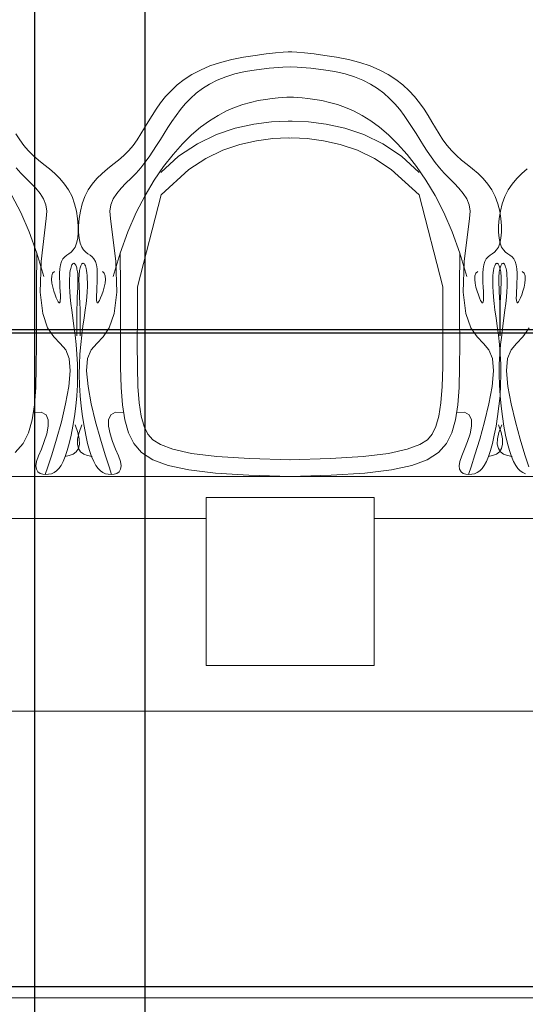
# Model space of a CAD drawing. Units: inches. Extents: x 1454 to 2136, y 626 to 1213.
# Tile 15 of 23: x 1654 to 1678, y 1095 to 1141. Entities that reach past the tile are written whole.
import ezdxf

# ---------------------------------------------------------------- set-up
doc = ezdxf.new("R2010")
doc.units = ezdxf.units.IN
doc.header["$MEASUREMENT"] = 0
for name, color, linetype, lineweight in [('A-ANNO-DIMS', 2, 'Continuous', 18), ('A-FURN-PATT', 252, 'Continuous', 13), ('conference', 41, 'Continuous', 18)]:
    doc.layers.add(name, color=color, linetype=linetype, lineweight=lineweight)
doc.styles.get("Standard").update_dxf_attribs({"font": 'arial.ttf'})
doc.dimstyles.get("Standard").update_dxf_attribs({"dimtxt": 4, "dimasz": 0.18, "dimexe": 0.18, "dimexo": 0.0625, "dimgap": 0.09, "dimtad": 0, "dimtih": 1, "dimtoh": 1, "dimdec": 0, "dimrnd": 6, "dimzin": 0, "dimdsep": 46, "dimlunit": 3, "dimtxsty": 'Standard', "dimcen": 0.09, "dimadec": 0, "dimazin": 0, "dimtfac": 1, "dimtdec": 0, "dimtofl": 0, "dimtmove": 0, "dimatfit": 3, "dimfxl": 1, "dimtolj": 1, "dimtzin": 0, "dimarcsym": 0})

# ---------------------------------------------------------------- blocks, each defined once
blk = doc.blocks.new('ОГ52_на12персон_стол2800х900')
for p, q in [((420.4, 772.5), (433.9, 776)), ((433.9, 776), (448, 778.8)), ((448, 778.8), (461.8, 780.9)), ((461.8, 780.9), (474.8, 782.6)), ((474.8, 782.6), (486.2, 783.7)), ((486.2, 783.7), (495.2, 784.5)), ((495.2, 784.5), (501.2, 784.9)), ((501.2, 784.9), (503.4, 785)), ((505.6, 784.9), (503.4, 785)), ((511.5, 784.5), (505.6, 784.9)), ((520.6, 783.7), (511.5, 784.5)), ((531.9, 782.6), (520.6, 783.7)), ((544.9, 780.9), (531.9, 782.6)), ((558.8, 778.8), (544.9, 780.9)), ((572.8, 776), (558.8, 778.8)), ((586.4, 772.5), (572.8, 776)), ((386.5, 758), (396.6, 763.4)), ((396.6, 763.4), (407.9, 768.3)), ((407.9, 768.3), (420.4, 772.5)), ((450.1, 761.5), (463.6, 763.8)), ((463.6, 763.8), (478.4, 765.6)), ((478.4, 765.6), (494.8, 766.8)), ((494.8, 766.8), (503.4, 767.1)), ((512, 766.8), (503.4, 767.1)), ((528.3, 765.6), (512, 766.8)), ((543.1, 763.8), (528.3, 765.6)), ((556.7, 761.5), (543.1, 763.8)), ((598.8, 768.3), (586.4, 772.5)), ((610.1, 763.4), (598.8, 768.3)), ((620.3, 758), (610.1, 763.4)), ((369, 745.6), (377.3, 752)), ((377.3, 752), (386.5, 758)), ((407.5, 746.6), (416.6, 751.2)), ((416.6, 751.2), (426.7, 755.2)), ((426.7, 755.2), (437.8, 758.7)), ((437.8, 758.7), (450.1, 761.5)), ((568.9, 758.7), (556.7, 761.5)), ((580, 755.2), (568.9, 758.7)), ((590.1, 751.2), (580, 755.2)), ((599.2, 746.6), (590.1, 751.2)), ((629.5, 752), (620.3, 758)), ((637.7, 745.6), (629.5, 752)), ((355, 731.7), (361.6, 738.8)), ((361.6, 738.8), (369, 745.6)), ((391.7, 735.7), (399.2, 741.4)), ((399.2, 741.4), (407.5, 746.6)), ((607.5, 741.4), (599.2, 746.6)), ((615, 735.7), (607.5, 741.4)), ((645.1, 738.8), (637.7, 745.6)), ((651.7, 731.7), (645.1, 738.8)), ((349.1, 724.4), (355, 731.7)), ((378.6, 723.1), (384.9, 729.6)), ((384.9, 729.6), (391.7, 735.7)), ((456.3, 724.9), (465.4, 727)), ((465.4, 727), (474.1, 728.5)), ((474.1, 728.5), (482, 729.6)), ((482, 729.6), (489.1, 730.4)), ((489.1, 730.4), (494.9, 730.8)), ((494.9, 730.8), (499.4, 731)), ((499.4, 731), (502.3, 731.1)), ((502.3, 731.1), (503.4, 731.1)), ((504.4, 731.1), (503.4, 731.1)), ((507.3, 731), (504.4, 731.1)), ((511.8, 730.8), (507.3, 731)), ((517.7, 730.4), (511.8, 730.8)), ((524.7, 729.6), (517.7, 730.4)), ((532.7, 728.5), (524.7, 729.6)), ((541.3, 727), (532.7, 728.5)), ((550.4, 724.9), (541.3, 727)), ((621.9, 729.6), (615, 735.7)), ((628.1, 723.1), (621.9, 729.6)), ((657.6, 724.4), (651.7, 731.7)), ((339, 709.4), (343.8, 716.9)), ((343.8, 716.9), (349.1, 724.4)), ((367.6, 709.3), (372.9, 716.3)), ((372.9, 716.3), (378.6, 723.1)), ((427.6, 714.7), (437.4, 718.9)), ((437.4, 718.9), (447, 722.3)), ((447, 722.3), (456.3, 724.9)), ((559.7, 722.3), (550.4, 724.9)), ((569.3, 718.9), (559.7, 722.3)), ((579.1, 714.7), (569.3, 718.9)), ((633.9, 716.3), (628.1, 723.1)), ((639.2, 709.3), (633.9, 716.3)), ((662.9, 716.9), (657.6, 724.4)), ((667.7, 709.4), (662.9, 716.9)), ((334.5, 701.9), (339, 709.4)), ((362.6, 702.2), (367.6, 709.3)), ((407.4, 703), (417.6, 709.4)), ((417.6, 709.4), (427.6, 714.7)), ((589.1, 709.4), (579.1, 714.7)), ((599.4, 703), (589.1, 709.4)), ((644.1, 702.2), (639.2, 709.3)), ((672.2, 701.9), (667.7, 709.4)), ((325.8, 687.3), (330.2, 694.5)), ((330.2, 694.5), (334.5, 701.9)), ((353.4, 687.9), (357.9, 695)), ((357.9, 695), (362.6, 702.2)), ((386.2, 686.1), (396.9, 695.3)), ((396.9, 695.3), (407.4, 703)), ((415.6, 686.5), (438.1, 694.2)), ((438.1, 694.2), (460.2, 699)), ((460.2, 699), (481.3, 701.6)), ((481.3, 701.6), (501, 702.5)), ((501, 702.5), (503.4, 702.4)), ((505.7, 702.5), (503.4, 702.4)), ((525.4, 701.6), (505.7, 702.5)), ((546.5, 699), (525.4, 701.6)), ((568.6, 694.2), (546.5, 699)), ((591.2, 686.5), (568.6, 694.2)), ((609.9, 695.3), (599.4, 703)), ((620.6, 686.1), (609.9, 695.3)), ((648.8, 695), (644.1, 702.2)), ((653.4, 687.9), (648.8, 695)), ((676.6, 694.5), (672.2, 701.9)), ((680.9, 687.3), (676.6, 694.5)), ((181.4, 680.3), (176.9, 687.3)), ((186.3, 673.7), (181.4, 680.3)), ((316.5, 673.7), (321.3, 680.3)), ((321.3, 680.3), (325.8, 687.3)), ((344.5, 673.7), (348.9, 680.7)), ((348.9, 680.7), (353.4, 687.9)), ((375.2, 675.4), (386.2, 686.1)), ((393, 675.6), (415.6, 686.5)), ((463.6, 679.3), (483, 681.7)), ((483, 681.7), (501.3, 682.5)), ((501.3, 682.5), (503, 682.4)), ((505.5, 682.5), (503.8, 682.4)), ((523.8, 681.7), (505.5, 682.5)), ((543.1, 679.3), (523.8, 681.7)), ((613.8, 675.6), (591.2, 686.5)), ((631.5, 675.4), (620.6, 686.1)), ((657.8, 680.7), (653.4, 687.9)), ((662.2, 673.7), (657.8, 680.7)), ((685.4, 680.3), (680.9, 687.3)), ((690.3, 673.7), (685.4, 680.3)), ((191.6, 667.5), (186.3, 673.7)), ((311.2, 667.5), (316.5, 673.7)), ((340.1, 666.7), (344.5, 673.7)), ((364, 663), (375.2, 675.4)), ((370.7, 660.8), (393, 675.6)), ((423.2, 668), (443.5, 674.9)), ((443.5, 674.9), (463.6, 679.3)), ((563.2, 674.9), (543.1, 679.3)), ((583.6, 668), (563.2, 674.9)), ((636, 660.8), (613.8, 675.6)), ((642.7, 663), (631.5, 675.4)), ((666.7, 666.7), (662.2, 673.7)), ((695.6, 667.5), (690.3, 673.7)), ((197.4, 661.7), (191.6, 667.5)), ((203.7, 656.2), (197.4, 661.7)), ((299, 656.2), (305.3, 661.7)), ((305.3, 661.7), (311.2, 667.5)), ((330.6, 653.3), (335.5, 659.9)), ((335.5, 659.9), (340.1, 666.7)), ((349.4, 641.6), (370.7, 660.8)), ((352.8, 648.7), (364, 663)), ((383, 644.9), (402.9, 658.2)), ((402.9, 658.2), (423.2, 668)), ((603.8, 658.2), (583.6, 668)), ((623.7, 644.9), (603.8, 658.2)), ((657.3, 641.6), (636, 660.8)), ((654, 648.7), (642.7, 663)), ((671.3, 659.9), (666.7, 666.7)), ((676.1, 653.3), (671.3, 659.9)), ((701.4, 661.7), (695.6, 667.5)), ((707.7, 656.2), (701.4, 661.7)), ((182.8, 640.6), (177.3, 646.8)), ((210.2, 650.9), (203.7, 656.2)), ((216.8, 645.6), (210.2, 650.9)), ((223.3, 640.1), (216.8, 645.6)), ((279.5, 640.1), (285.9, 645.6)), ((285.9, 645.6), (292.5, 650.9)), ((292.5, 650.9), (299, 656.2)), ((320, 640.6), (325.5, 646.8)), ((325.5, 646.8), (330.6, 653.3)), ((341.6, 632.4), (352.8, 648.7)), ((349.8, 615), (383, 644.9)), ((657, 615), (623.7, 644.9)), ((665.2, 632.4), (654, 648.7)), ((681.3, 646.8), (676.1, 653.3)), ((686.8, 640.6), (681.3, 646.8)), ((714.2, 650.9), (707.7, 656.2)), ((720.8, 645.6), (714.2, 650.9)), ((727.3, 640.1), (720.8, 645.6)), ((779.5, 640.1), (785.9, 645.6)), ((188.7, 634.6), (182.8, 640.6)), ((194.7, 628.7), (188.7, 634.6)), ((229.3, 634.2), (223.3, 640.1)), ((234.9, 627.7), (229.3, 634.2)), ((267.8, 627.7), (273.4, 634.2)), ((273.4, 634.2), (279.5, 640.1)), ((308, 628.7), (314.1, 634.6)), ((314.1, 634.6), (320, 640.6)), ((692.7, 634.6), (686.8, 640.6)), ((698.7, 628.7), (692.7, 634.6)), ((733.4, 634.2), (727.3, 640.1)), ((738.9, 627.7), (733.4, 634.2)), ((767.8, 627.7), (773.4, 634.2)), ((773.4, 634.2), (779.5, 640.1)), ((200.5, 622.8), (194.7, 628.7)), ((205.6, 616.6), (200.5, 622.8)), ((239.7, 620.6), (234.9, 627.7)), ((263, 620.6), (267.8, 627.7)), ((297.1, 616.6), (302.3, 622.8)), ((302.3, 622.8), (308, 628.7)), ((330.7, 614.1), (341.6, 632.4)), ((676.1, 614.1), (665.2, 632.4)), ((704.5, 622.8), (698.7, 628.7)), ((709.6, 616.6), (704.5, 622.8)), ((743.7, 620.6), (738.9, 627.7)), ((763, 620.6), (767.8, 627.7)), ((182.6, 593.6), (172.1, 614.1)), ((209.8, 610.1), (205.6, 616.6)), ((212.7, 603), (209.8, 610.1)), ((243.7, 612.7), (239.7, 620.6)), ((246.7, 604.2), (243.7, 612.7)), ((256, 604.2), (259.1, 612.7)), ((259.1, 612.7), (263, 620.6)), ((290, 603), (292.9, 610.1)), ((292.9, 610.1), (297.1, 616.6)), ((320.1, 593.6), (330.7, 614.1)), ((349.8, 615), (321.5, 505.2)), ((657, 615), (685.3, 505.2)), ((686.6, 593.6), (676.1, 614.1)), ((713.8, 610.1), (709.6, 616.6)), ((716.7, 603), (713.8, 610.1)), ((747.7, 612.7), (743.7, 620.6)), ((750.7, 604.2), (747.7, 612.7)), ((756, 604.2), (759.1, 612.7)), ((759.1, 612.7), (763, 620.6)), ((213.9, 595.2), (212.7, 603)), ((249, 595.4), (246.7, 604.2)), ((253.8, 595.4), (256, 604.2)), ((288.8, 595.2), (290, 603)), ((717.9, 595.2), (716.7, 603)), ((753, 595.4), (750.7, 604.2)), ((753.8, 595.4), (756, 604.2)), ((192.5, 570.7), (182.6, 593.6)), ((213.1, 586.5), (206.8, 535.5)), ((213.1, 586.5), (213.9, 595.2)), ((250.4, 586.6), (249, 595.4)), ((251.1, 578.1), (250.4, 586.6)), ((251.6, 578.1), (252.3, 586.6)), ((252.3, 586.6), (253.8, 595.4)), ((289.6, 586.5), (288.8, 595.2)), ((289.6, 586.5), (296, 535.5)), ((310.2, 570.7), (320.1, 593.6)), ((696.5, 570.7), (686.6, 593.6)), ((717.1, 586.5), (710.8, 535.5)), ((717.1, 586.5), (717.9, 595.2)), ((751.6, 578.1), (752.3, 586.6)), ((752.3, 586.6), (753.8, 595.4)), ((754.4, 586.6), (753, 595.4)), ((755.1, 578.1), (754.4, 586.6)), ((251.1, 570.2), (251.1, 578.1)), ((251.6, 570.2), (251.6, 578.1)), ((751.6, 570.2), (751.6, 578.1)), ((755.1, 570.2), (755.1, 578.1)), ((201.7, 545.4), (192.5, 570.7)), ((249.2, 557.2), (250.5, 563.1)), ((250.5, 563.1), (251.1, 570.2)), ((252.3, 563.1), (251.6, 570.2)), ((253.5, 557.2), (252.3, 563.1)), ((301, 545.4), (310.2, 570.7)), ((705.7, 545.4), (696.5, 570.7)), ((752.3, 563.1), (751.6, 570.2)), ((753.5, 557.2), (752.3, 563.1)), ((753.2, 557.2), (754.5, 563.1)), ((754.5, 563.1), (755.1, 570.2)), ((245.2, 549.3), (247.4, 552.7)), ((247.4, 552.7), (249.2, 557.2)), ((255.3, 552.7), (253.5, 557.2)), ((257.5, 549.3), (255.3, 552.7)), ((749.2, 549.3), (751.4, 552.7)), ((751.4, 552.7), (753.2, 557.2)), ((755.3, 552.7), (753.5, 557.2)), ((757.5, 549.3), (755.3, 552.7)), ((201.7, 545.4), (201.3, 505.1)), ((210, 517.6), (201.7, 545.4)), ((232.9, 538.5), (235.1, 540.8)), ((235.1, 540.8), (237.5, 542.8)), ((237.5, 542.8), (240.1, 544.6)), ((240.1, 544.6), (242.7, 546.7)), ((242.7, 546.7), (245.2, 549.3)), ((260, 546.7), (257.5, 549.3)), ((262.6, 544.6), (260, 546.7)), ((265.2, 542.8), (262.6, 544.6)), ((267.7, 540.8), (265.2, 542.8)), ((269.8, 538.5), (267.7, 540.8)), ((292.7, 517.6), (301, 545.4)), ((301, 545.4), (301.5, 505.1)), ((705.7, 545.4), (705.3, 505.1)), ((714, 517.6), (705.7, 545.4)), ((736.9, 538.5), (739.1, 540.8)), ((739.1, 540.8), (741.5, 542.8)), ((741.5, 542.8), (744.1, 544.6)), ((744.1, 544.6), (746.7, 546.7)), ((746.7, 546.7), (749.2, 549.3)), ((760, 546.7), (757.5, 549.3)), ((762.6, 544.6), (760, 546.7)), ((765.2, 542.8), (762.6, 544.6)), ((767.7, 540.8), (765.2, 542.8)), ((769.8, 538.5), (767.7, 540.8)), ((206.8, 535.5), (205.7, 498.8)), ((229.3, 526.8), (230, 531.5)), ((230, 531.5), (231.2, 535.5)), ((231.2, 535.5), (232.9, 538.5)), ((242.2, 527), (242.6, 528.8)), ((242.6, 528.8), (243.1, 530.3)), ((243.1, 530.3), (243.6, 531.5)), ((243.6, 531.5), (244.1, 532.3)), ((244.1, 532.3), (244.7, 532.9)), ((244.7, 532.9), (245.2, 533.2)), ((245.2, 533.2), (245.7, 533.3)), ((245.7, 533.3), (246.2, 533.2)), ((246.2, 533.2), (246.7, 533)), ((246.7, 533), (247.2, 532.5)), ((247.2, 532.5), (247.6, 531.9)), ((247.6, 531.9), (248.1, 531.1)), ((248.1, 531.1), (248.5, 530.2)), ((248.5, 530.2), (248.9, 529.1)), ((248.9, 529.1), (249.3, 527.9)), ((249.3, 527.9), (249.6, 526.5)), ((253.5, 527.9), (253.1, 526.5)), ((253.8, 529.1), (253.5, 527.9)), ((254.2, 530.2), (253.8, 529.1)), ((254.7, 531.1), (254.2, 530.2)), ((255.1, 531.9), (254.7, 531.1)), ((255.6, 532.5), (255.1, 531.9)), ((256, 533), (255.6, 532.5)), ((256.5, 533.2), (256, 533)), ((257, 533.3), (256.5, 533.2)), ((257.6, 533.2), (257, 533.3)), ((258.1, 532.9), (257.6, 533.2)), ((258.6, 532.3), (258.1, 532.9)), ((259.1, 531.5), (258.6, 532.3)), ((259.6, 530.3), (259.1, 531.5)), ((260.1, 528.8), (259.6, 530.3)), ((260.6, 527), (260.1, 528.8)), ((271.6, 535.5), (269.8, 538.5)), ((272.8, 531.5), (271.6, 535.5)), ((273.5, 526.8), (272.8, 531.5)), ((296, 535.5), (297, 498.8)), ((710.8, 535.5), (709.7, 498.8)), ((733.3, 526.8), (734, 531.5)), ((734, 531.5), (735.2, 535.5)), ((735.2, 535.5), (736.9, 538.5)), ((746.2, 527), (746.6, 528.8)), ((746.6, 528.8), (747.1, 530.3)), ((747.1, 530.3), (747.6, 531.5)), ((747.6, 531.5), (748.1, 532.3)), ((748.1, 532.3), (748.7, 532.9)), ((748.7, 532.9), (749.2, 533.2)), ((749.2, 533.2), (749.7, 533.3)), ((749.7, 533.3), (750.2, 533.2)), ((750.2, 533.2), (750.7, 533)), ((750.7, 533), (751.2, 532.5)), ((751.2, 532.5), (751.6, 531.9)), ((751.6, 531.9), (752.1, 531.1)), ((752.1, 531.1), (752.5, 530.2)), ((752.5, 530.2), (752.9, 529.1)), ((752.9, 529.1), (753.3, 527.9)), ((753.5, 527.9), (753.1, 526.5)), ((753.3, 527.9), (753.6, 526.5)), ((753.8, 529.1), (753.5, 527.9)), ((754.2, 530.2), (753.8, 529.1)), ((754.7, 531.1), (754.2, 530.2)), ((755.1, 531.9), (754.7, 531.1)), ((755.6, 532.5), (755.1, 531.9)), ((756, 533), (755.6, 532.5)), ((756.5, 533.2), (756, 533)), ((757, 533.3), (756.5, 533.2)), ((757.6, 533.2), (757, 533.3)), ((758.1, 532.9), (757.6, 533.2)), ((758.6, 532.3), (758.1, 532.9)), ((759.1, 531.5), (758.6, 532.3)), ((759.6, 530.3), (759.1, 531.5)), ((760.1, 528.8), (759.6, 530.3)), ((760.6, 527), (760.1, 528.8)), ((771.6, 535.5), (769.8, 538.5)), ((772.8, 531.5), (771.6, 535.5)), ((773.5, 526.8), (772.8, 531.5)), ((219.5, 518.2), (219.3, 514.2)), ((220.6, 521.4), (219.5, 518.2)), ((222.8, 523.4), (220.6, 521.4)), ((228.9, 521.5), (229.3, 526.8)), ((228.9, 516), (228.9, 521.5)), ((229.1, 510.3), (228.9, 516)), ((240.8, 514.9), (241, 518.7)), ((241, 518.7), (241.3, 521.9)), ((241.3, 521.9), (241.7, 524.7)), ((241.7, 524.7), (242.2, 527)), ((249.6, 526.5), (250, 524.9)), ((250, 524.9), (250.2, 523.1)), ((250.2, 523.1), (250.5, 521)), ((250.5, 521), (250.6, 518.5)), ((250.6, 518.5), (250.7, 515.7)), ((252.1, 518.5), (252, 515.7)), ((252.3, 521), (252.1, 518.5)), ((252.5, 523.1), (252.3, 521)), ((252.8, 524.9), (252.5, 523.1)), ((253.1, 526.5), (252.8, 524.9)), ((261, 524.7), (260.6, 527)), ((261.4, 521.9), (261, 524.7)), ((261.7, 518.7), (261.4, 521.9)), ((261.9, 514.9), (261.7, 518.7)), ((273.8, 521.5), (273.5, 526.8)), ((273.6, 510.3), (273.8, 516)), ((273.8, 516), (273.8, 521.5)), ((279.9, 523.4), (282.1, 521.4)), ((282.1, 521.4), (283.2, 518.2)), ((283.2, 518.2), (283.5, 514.2)), ((723.5, 518.2), (723.3, 514.2)), ((724.6, 521.4), (723.5, 518.2)), ((726.8, 523.4), (724.6, 521.4)), ((732.9, 521.5), (733.3, 526.8)), ((732.9, 516), (732.9, 521.5)), ((733.1, 510.3), (732.9, 516)), ((744.8, 514.9), (745, 518.7)), ((745, 518.7), (745.3, 521.9)), ((745.3, 521.9), (745.7, 524.7)), ((745.7, 524.7), (746.2, 527)), ((752.1, 518.5), (752, 515.7)), ((752.3, 521), (752.1, 518.5)), ((752.5, 523.1), (752.3, 521)), ((752.8, 524.9), (752.5, 523.1)), ((753.1, 526.5), (752.8, 524.9)), ((753.6, 526.5), (754, 524.9)), ((754, 524.9), (754.2, 523.1)), ((754.2, 523.1), (754.5, 521)), ((754.5, 521), (754.6, 518.5)), ((754.6, 518.5), (754.7, 515.7)), ((761, 524.7), (760.6, 527)), ((761.4, 521.9), (761, 524.7)), ((761.7, 518.7), (761.4, 521.9)), ((761.9, 514.9), (761.7, 518.7)), ((773.8, 521.5), (773.5, 526.8)), ((773.6, 510.3), (773.8, 516)), ((773.8, 516), (773.8, 521.5)), ((779.9, 523.4), (782.1, 521.4)), ((782.1, 521.4), (783.2, 518.2)), ((783.2, 518.2), (783.5, 514.2)), ((201.3, 505.1), (201.3, 469.2)), ((219.3, 514.2), (219.7, 509.6)), ((219.7, 509.6), (220.7, 504.8)), ((220.7, 504.8), (222.1, 500.1)), ((229.4, 504.9), (229.1, 510.3)), ((229.7, 499.8), (229.4, 504.9)), ((240.7, 510.5), (240.8, 514.9)), ((240.8, 505.4), (240.7, 510.5)), ((241.1, 499.6), (240.8, 505.4)), ((250.6, 508.5), (250.5, 504)), ((250.7, 512.3), (250.6, 508.5)), ((250.7, 515.7), (250.7, 512.3)), ((252, 515.7), (252, 512.3)), ((252, 512.3), (252.1, 508.5)), ((252.1, 508.5), (252.3, 504)), ((261.7, 499.6), (262, 505.4)), ((262, 510.5), (261.9, 514.9)), ((262, 505.4), (262, 510.5)), ((273.1, 499.8), (273.4, 504.9)), ((273.4, 504.9), (273.6, 510.3)), ((282, 504.8), (280.7, 500.1)), ((283, 509.6), (282, 504.8)), ((283.5, 514.2), (283, 509.6)), ((301.5, 505.1), (301.5, 469.2)), ((321.5, 505.2), (321.5, 469.2)), ((685.3, 505.2), (685.3, 469.2)), ((705.3, 505.1), (705.3, 469.2)), ((723.3, 514.2), (723.7, 509.6)), ((723.7, 509.6), (724.7, 504.8)), ((724.7, 504.8), (726.1, 500.1)), ((733.4, 504.9), (733.1, 510.3)), ((733.7, 499.8), (733.4, 504.9)), ((744.7, 510.5), (744.8, 514.9)), ((744.8, 505.4), (744.7, 510.5)), ((745.1, 499.6), (744.8, 505.4)), ((752, 515.7), (752, 512.3)), ((752, 512.3), (752.1, 508.5)), ((752.1, 508.5), (752.3, 504)), ((754.6, 508.5), (754.5, 504)), ((754.7, 512.3), (754.6, 508.5)), ((754.7, 515.7), (754.7, 512.3)), ((761.7, 499.6), (762, 505.4)), ((762, 510.5), (761.9, 514.9)), ((762, 505.4), (762, 510.5)), ((773.1, 499.8), (773.4, 504.9)), ((773.4, 504.9), (773.6, 510.3)), ((782, 504.8), (780.7, 500.1)), ((783, 509.6), (782, 504.8)), ((783.5, 514.2), (783, 509.6)), ((205.7, 498.8), (208.8, 473.4)), ((222.1, 500.1), (223.6, 495.7)), ((223.6, 495.7), (225, 492)), ((229.9, 495.4), (229.7, 499.8)), ((229.9, 491.8), (229.9, 495.4)), ((241.6, 493.1), (241.1, 499.6)), ((242.4, 485.6), (241.6, 493.1)), ((249.9, 493), (249.7, 486.1)), ((250.2, 498.9), (249.9, 493)), ((250.5, 504), (250.2, 498.9)), ((252.3, 504), (252.5, 498.9)), ((252.5, 498.9), (252.8, 493)), ((252.8, 493), (253.1, 486.1)), ((260.4, 485.6), (261.2, 493.1)), ((261.2, 493.1), (261.7, 499.6)), ((272.8, 491.8), (272.9, 495.4)), ((272.9, 495.4), (273.1, 499.8)), ((279.2, 495.7), (277.7, 492)), ((280.7, 500.1), (279.2, 495.7)), ((297, 498.8), (294, 473.4)), ((709.7, 498.8), (712.8, 473.4)), ((726.1, 500.1), (727.6, 495.7)), ((727.6, 495.7), (729, 492)), ((733.9, 495.4), (733.7, 499.8)), ((733.9, 491.8), (733.9, 495.4)), ((745.6, 493.1), (745.1, 499.6)), ((746.4, 485.6), (745.6, 493.1)), ((752.3, 504), (752.5, 498.9)), ((752.5, 498.9), (752.8, 493)), ((752.8, 493), (753.1, 486.1)), ((753.9, 493), (753.7, 486.1)), ((754.2, 498.9), (753.9, 493)), ((754.5, 504), (754.2, 498.9)), ((760.4, 485.6), (761.2, 493.1)), ((761.2, 493.1), (761.7, 499.6)), ((772.8, 491.8), (772.9, 495.4)), ((772.9, 495.4), (773.1, 499.8)), ((779.2, 495.7), (777.7, 492)), ((780.7, 500.1), (779.2, 495.7)), ((225, 492), (226.3, 489.2)), ((226.3, 489.2), (227.4, 487.3)), ((227.4, 487.3), (228.3, 486.4)), ((228.3, 486.4), (229, 486.4)), ((229, 486.4), (229.5, 487.3)), ((229.5, 487.3), (229.8, 489.1)), ((229.8, 489.1), (229.9, 491.8)), ((243.4, 477.3), (242.4, 485.6)), ((249.7, 486.1), (249.4, 478.2)), ((253.1, 486.1), (253.3, 478.2)), ((259.3, 477.3), (260.4, 485.6)), ((272.9, 489.1), (272.8, 491.8)), ((273.3, 487.3), (272.9, 489.1)), ((273.8, 486.4), (273.3, 487.3)), ((274.4, 486.4), (273.8, 486.4)), ((275.3, 487.3), (274.4, 486.4)), ((276.4, 489.2), (275.3, 487.3)), ((277.7, 492), (276.4, 489.2)), ((729, 492), (730.3, 489.2)), ((730.3, 489.2), (731.4, 487.3)), ((731.4, 487.3), (732.3, 486.4)), ((732.3, 486.4), (733, 486.4)), ((733, 486.4), (733.5, 487.3)), ((733.5, 487.3), (733.8, 489.1)), ((733.8, 489.1), (733.9, 491.8)), ((747.4, 477.3), (746.4, 485.6)), ((753.1, 486.1), (753.3, 478.2)), ((753.7, 486.1), (753.4, 478.2)), ((759.3, 477.3), (760.4, 485.6)), ((772.9, 489.1), (772.8, 491.8)), ((773.3, 487.3), (772.9, 489.1)), ((773.8, 486.4), (773.3, 487.3)), ((774.4, 486.4), (773.8, 486.4)), ((775.3, 487.3), (774.4, 486.4)), ((776.4, 489.2), (775.3, 487.3)), ((777.7, 492), (776.4, 489.2)), ((201.3, 469.2), (201.4, 437.5)), ((208.8, 473.4), (214.6, 456.6)), ((244.7, 468.2), (243.4, 477.3)), ((249.4, 478.2), (249.3, 469.2)), ((249.3, 469.2), (249.3, 458.8)), ((253.3, 478.2), (253.4, 469.2)), ((253.4, 469.2), (253.5, 458.8)), ((258, 468.2), (259.3, 477.3)), ((294, 473.4), (288.1, 456.6)), ((301.5, 469.2), (301.4, 437.5)), ((321.5, 469.2), (321.4, 437.6)), ((685.3, 469.2), (685.4, 437.6)), ((705.3, 469.2), (705.4, 437.5)), ((712.8, 473.4), (718.6, 456.6)), ((748.7, 468.2), (747.4, 477.3)), ((753.3, 478.2), (753.4, 469.2)), ((753.4, 478.2), (753.3, 469.2)), ((753.3, 469.2), (753.3, 458.8)), ((753.4, 469.2), (753.5, 458.8)), ((758, 468.2), (759.3, 477.3)), ((246, 458.3), (244.7, 468.2)), ((247.4, 447.8), (246, 458.3)), ((249.3, 458.8), (249.4, 447.1)), ((253.5, 458.8), (253.3, 447.1)), ((255.4, 447.8), (256.7, 458.3)), ((256.7, 458.3), (258, 468.2)), ((750, 458.3), (748.7, 468.2)), ((751.4, 447.8), (750, 458.3)), ((753.5, 458.8), (753.3, 447.1)), ((753.3, 458.8), (753.4, 447.1)), ((755.4, 447.8), (756.7, 458.3)), ((756.7, 458.3), (758, 468.2)), ((214.6, 456.6), (222, 445.7)), ((222, 445.7), (229.6, 437.8)), ((248.6, 436.7), (247.4, 447.8)), ((254.1, 436.7), (255.4, 447.8)), ((280.7, 445.7), (273.1, 437.8)), ((288.1, 456.6), (280.7, 445.7)), ((718.6, 456.6), (726, 445.7)), ((726, 445.7), (733.6, 437.8)), ((752.6, 436.7), (751.4, 447.8)), ((754.1, 436.7), (755.4, 447.8)), ((780.7, 445.7), (773.1, 437.8)), ((788.1, 456.6), (780.7, 445.7)), ((201.4, 437.5), (201.2, 409.8)), ((229.6, 437.8), (236.2, 430.2)), ((249.6, 425.1), (248.6, 436.7)), ((253.1, 425.1), (254.1, 436.7)), ((273.1, 437.8), (266.5, 430.2)), ((301.4, 437.5), (301.5, 409.8)), ((321.4, 437.6), (321.5, 410.1)), ((685.4, 437.6), (685.3, 410.1)), ((705.4, 437.5), (705.3, 409.8)), ((733.6, 437.8), (740.2, 430.2)), ((753.6, 425.1), (752.6, 436.7)), ((753.1, 425.1), (754.1, 436.7)), ((773.1, 437.8), (766.5, 430.2)), ((236.2, 430.2), (240.5, 420)), ((250.2, 413.1), (249.6, 425.1)), ((252.5, 413.1), (253.1, 425.1)), ((266.5, 430.2), (262.2, 420)), ((740.2, 430.2), (744.5, 420)), ((752.5, 413.1), (753.1, 425.1)), ((754.2, 413.1), (753.6, 425.1)), ((766.5, 430.2), (762.2, 420)), ((240.5, 420), (241.6, 405.3)), ((250.4, 400.7), (250.2, 413.1)), ((252.3, 400.7), (252.5, 413.1)), ((262.2, 420), (261.1, 405.3)), ((744.5, 420), (745.6, 405.3)), ((752.3, 400.7), (752.5, 413.1)), ((754.4, 400.7), (754.2, 413.1)), ((762.2, 420), (761.1, 405.3)), ((201.2, 409.8), (200.6, 385.6)), ((241.6, 405.3), (239.9, 386.7)), ((250.1, 388.2), (250.4, 400.7)), ((252.6, 388.2), (252.3, 400.7)), ((261.1, 405.3), (262.8, 386.7)), ((301.5, 409.8), (302.2, 385.6)), ((321.5, 410.1), (322.1, 386.6)), ((685.3, 410.1), (684.6, 386.6)), ((705.3, 409.8), (704.6, 385.6)), ((745.6, 405.3), (743.9, 386.7)), ((752.6, 388.2), (752.3, 400.7)), ((754.1, 388.2), (754.4, 400.7)), ((761.1, 405.3), (762.8, 386.7)), ((249.3, 375.5), (250.1, 388.2)), ((253.4, 375.5), (252.6, 388.2)), ((753.4, 375.5), (752.6, 388.2)), ((753.4, 375.5), (754.1, 388.2)), ((200.6, 385.6), (199, 364.7)), ((239.9, 386.7), (236.1, 366)), ((248.1, 363), (249.3, 375.5)), ((254.6, 363), (253.4, 375.5)), ((262.8, 386.7), (266.6, 366)), ((302.2, 385.6), (303.7, 364.7)), ((322.1, 386.6), (323.6, 367)), ((684.6, 386.6), (683.1, 367)), ((704.6, 385.6), (703, 364.7)), ((743.9, 386.7), (740.1, 366)), ((752.1, 363), (753.4, 375.5)), ((754.6, 363), (753.4, 375.5)), ((762.8, 386.7), (766.6, 366)), ((199, 364.7), (196.2, 346.8)), ((236.1, 366), (231, 344.5)), ((266.6, 366), (271.8, 344.5)), ((303.7, 364.7), (306.5, 346.8)), ((323.6, 367), (326.1, 351.1)), ((683.1, 367), (680.6, 351.1)), ((703, 364.7), (700.2, 346.8)), ((740.1, 366), (735, 344.5)), ((766.6, 366), (771.8, 344.5)), ((207.1, 356.1), (197.6, 355.7)), ((212.8, 353), (207.1, 356.1)), ((215.4, 347.1), (212.8, 353)), ((246.6, 350.9), (248.1, 363)), ((256.2, 350.9), (254.6, 363)), ((287.3, 347.1), (289.9, 353)), ((289.9, 353), (295.6, 356.1)), ((295.6, 356.1), (305.1, 355.7)), ((711.1, 356.1), (701.6, 355.7)), ((716.8, 353), (711.1, 356.1)), ((719.4, 347.1), (716.8, 353)), ((750.6, 350.9), (752.1, 363)), ((756.2, 350.9), (754.6, 363)), ((196.2, 346.8), (191.8, 331.5)), ((215.5, 339.3), (215.4, 347.1)), ((231, 344.5), (225.2, 323.8)), ((244.7, 339.4), (246.6, 350.9)), ((247.4, 341), (250.7, 331.8)), ((255.4, 341), (252.1, 331.8)), ((258, 339.4), (256.2, 350.9)), ((271.8, 344.5), (277.5, 323.8)), ((287.3, 339.3), (287.3, 347.1)), ((306.5, 346.8), (310.9, 331.5)), ((326.1, 351.1), (329.6, 338.8)), ((680.6, 351.1), (677.1, 338.8)), ((700.2, 346.8), (695.9, 331.5)), ((719.5, 339.3), (719.4, 347.1)), ((735, 344.5), (729.2, 323.8)), ((748.7, 339.4), (750.6, 350.9)), ((751.4, 341), (754.7, 331.8)), ((755.4, 341), (752.1, 331.8)), ((758, 339.4), (756.2, 350.9)), ((771.8, 344.5), (777.5, 323.8)), ((191.8, 331.5), (185.5, 318.7)), ((210.7, 321), (213.7, 330.3)), ((213.7, 330.3), (215.5, 339.3)), ((240.4, 318.9), (242.6, 328.7)), ((242.6, 328.7), (244.7, 339.4)), ((252.1, 331.8), (250.4, 324.1)), ((250.7, 331.8), (252.3, 324.1)), ((260.1, 328.7), (258, 339.4)), ((262.3, 318.9), (260.1, 328.7)), ((289.1, 330.3), (287.3, 339.3)), ((292, 321), (289.1, 330.3)), ((310.9, 331.5), (317.3, 318.7)), ((329.6, 338.8), (334, 329.9)), ((334, 329.9), (339.8, 323.3)), ((672.7, 329.9), (666.9, 323.3)), ((677.1, 338.8), (672.7, 329.9)), ((695.9, 331.5), (689.5, 318.7)), ((714.7, 321), (717.7, 330.3)), ((717.7, 330.3), (719.5, 339.3)), ((744.4, 318.9), (746.6, 328.7)), ((746.6, 328.7), (748.7, 339.4)), ((752.1, 331.8), (750.4, 324.1)), ((754.7, 331.8), (756.3, 324.1)), ((760.1, 328.7), (758, 339.4)), ((762.3, 318.9), (760.1, 328.7)), ((185.5, 318.7), (176.2, 308)), ((207.2, 312), (210.7, 321)), ((225.2, 323.8), (219.6, 305.4)), ((238.1, 310.4), (240.4, 318.9)), ((250.4, 324.1), (250.2, 317.8)), ((250.2, 317.8), (251.5, 312.9)), ((252.5, 317.8), (251.3, 312.9)), ((252.3, 324.1), (252.5, 317.8)), ((264.7, 310.4), (262.3, 318.9)), ((277.5, 323.8), (283.1, 305.4)), ((295.5, 312), (292, 321)), ((317.3, 318.7), (326.6, 308)), ((339.8, 323.3), (349, 317.4)), ((349, 317.4), (363.9, 311.8)), ((657.8, 317.4), (642.8, 311.8)), ((666.9, 323.3), (657.8, 317.4)), ((689.5, 318.7), (680.2, 308)), ((711.2, 312), (714.7, 321)), ((729.2, 323.8), (723.6, 305.4)), ((742.1, 310.4), (744.4, 318.9)), ((750.4, 324.1), (750.2, 317.8)), ((750.2, 317.8), (751.5, 312.9)), ((756.5, 317.8), (755.3, 312.9)), ((756.3, 324.1), (756.5, 317.8)), ((764.7, 310.4), (762.3, 318.9)), ((777.5, 323.8), (783.1, 305.4)), ((203.8, 304.2), (207.2, 312)), ((219.6, 305.4), (214.9, 291)), ((235.7, 303.2), (238.1, 310.4)), ((245.2, 306.2), (240.5, 304.3)), ((248.8, 309), (245.2, 306.2)), ((251.3, 312.9), (248.8, 309)), ((251.5, 312.9), (254, 309)), ((254, 309), (257.6, 306.2)), ((257.6, 306.2), (262.2, 304.3)), ((267.1, 303.2), (264.7, 310.4)), ((283.1, 305.4), (287.8, 291)), ((298.9, 304.2), (295.5, 312)), ((326.6, 308), (339.9, 299.4)), ((363.9, 311.8), (386.1, 307)), ((386.1, 307), (416.3, 303.4)), ((620.7, 307), (590.5, 303.4)), ((642.8, 311.8), (620.7, 307)), ((680.2, 308), (666.8, 299.4)), ((707.8, 304.2), (711.2, 312)), ((723.6, 305.4), (718.9, 291)), ((739.7, 303.2), (742.1, 310.4)), ((749.2, 306.2), (744.6, 304.3)), ((752.8, 309), (749.2, 306.2)), ((751.5, 312.9), (754, 309)), ((755.3, 312.9), (752.8, 309)), ((754, 309), (757.6, 306.2)), ((757.6, 306.2), (762.2, 304.3)), ((767.1, 303.2), (764.7, 310.4)), ((783.1, 305.4), (787.8, 291)), ((201.4, 297.4), (200.6, 292.1)), ((203.8, 304.2), (201.4, 297.4)), ((230.7, 292.5), (233.2, 297.3)), ((233.2, 297.3), (235.7, 303.2)), ((240.5, 304.3), (235.1, 303.1)), ((262.2, 304.3), (267.7, 303.1)), ((269.5, 297.3), (267.1, 303.2)), ((272.1, 292.5), (269.5, 297.3)), ((298.9, 304.2), (301.3, 297.4)), ((301.3, 297.4), (302.1, 292.1)), ((339.9, 299.4), (358.3, 292.5)), ((416.3, 303.4), (455.2, 300.9)), ((455.2, 300.9), (504, 299.3)), ((551.5, 300.9), (502.7, 299.3)), ((590.5, 303.4), (551.5, 300.9)), ((666.8, 299.4), (648.5, 292.5)), ((705.4, 297.4), (704.6, 292.1)), ((707.8, 304.2), (705.4, 297.4)), ((734.7, 292.5), (737.2, 297.3)), ((737.2, 297.3), (739.7, 303.2)), ((744.6, 304.3), (739.1, 303.1)), ((762.2, 304.3), (767.7, 303.1)), ((769.5, 297.3), (767.1, 303.2)), ((772.1, 292.5), (769.5, 297.3)), ((200.6, 292.1), (201.3, 288.1)), ((201.3, 288.1), (203, 285.1)), ((203, 285.1), (205.6, 283.2)), ((205.6, 283.2), (208.8, 282.2)), ((208.8, 282.2), (212.3, 281.8)), ((214.9, 291), (211.9, 281.9)), ((212.3, 281.8), (215.8, 282.1)), ((215.8, 282.1), (219.2, 282.8)), ((219.2, 282.8), (222.3, 284.1)), ((222.3, 284.1), (225.2, 286.1)), ((225.2, 286.1), (228, 288.8)), ((228, 288.8), (230.7, 292.5)), ((274.7, 288.8), (272.1, 292.5)), ((277.5, 286.1), (274.7, 288.8)), ((280.4, 284.1), (277.5, 286.1)), ((283.6, 282.8), (280.4, 284.1)), ((286.9, 282.1), (283.6, 282.8)), ((290.4, 281.8), (286.9, 282.1)), ((287.8, 291), (290.9, 281.9)), ((293.9, 282.2), (290.4, 281.8)), ((297.1, 283.2), (293.9, 282.2)), ((299.7, 285.1), (297.1, 283.2)), ((301.5, 288.1), (299.7, 285.1)), ((302.1, 292.1), (301.5, 288.1)), ((358.3, 292.5), (382.8, 287.3)), ((382.8, 287.3), (414.4, 283.5)), ((414.4, 283.5), (454.3, 280.9)), ((592.3, 283.5), (552.5, 280.9)), ((624, 287.3), (592.3, 283.5)), ((648.5, 292.5), (624, 287.3)), ((704.6, 292.1), (705.3, 288.1)), ((705.3, 288.1), (707, 285.1)), ((707, 285.1), (709.6, 283.2)), ((709.6, 283.2), (712.8, 282.2)), ((712.8, 282.2), (716.3, 281.8)), ((718.9, 291), (715.9, 281.9)), ((716.3, 281.8), (719.8, 282.1)), ((719.8, 282.1), (723.2, 282.8)), ((723.2, 282.8), (726.3, 284.1)), ((726.3, 284.1), (729.2, 286.1)), ((729.2, 286.1), (732, 288.8)), ((732, 288.8), (734.7, 292.5)), ((774.7, 288.8), (772.1, 292.5)), ((777.5, 286.1), (774.7, 288.8)), ((780.4, 284.1), (777.5, 286.1)), ((783.6, 282.8), (780.4, 284.1)), ((-1300, 279.3), (1300, 279.3)), ((454.3, 280.9), (503.4, 279.3)), ((552.5, 280.9), (503.4, 279.3)), ((403.4, 54.3), (403.4, 254.3)), ((403.4, 254.3), (603.4, 254.3)), ((603.4, 254.3), (603.4, 54.3)), ((403.4, 229.3), (96.6, 229.3)), ((603.4, 229.3), (903.4, 229.3)), ((603.4, 54.3), (403.4, 54.3)), ((1220.7, 0), (-1220.7, 0)), ((-1220.7, -341.4), (1220.7, -341.4))]:
    blk.add_line(p, q)
blk = doc.blocks.new('*D23')
at = {"layer": 'A-ANNO-DIMS', "color": 0, "lineweight": -2, "transparency": 16777216}
for p, q in [((1571.674, 1139.532), (1571.674, 1162.157)), ((1571.854, 1161.977), (1615.675, 1161.977)), ((1721.545, 1161.977), (1677.724, 1161.977)), ((1721.725, 1139.532), (1721.725, 1162.157))]:
    blk.add_line(p, q, dxfattribs=at)
at = {"layer": 'A-ANNO-DIMS', "color": 0, "transparency": 16777216}
for points in [[(1571.854, 1162.007), (1571.854, 1161.947), (1571.674, 1161.977)], [(1721.545, 1162.007), (1721.545, 1161.947), (1721.725, 1161.977)]]:
    blk.add_solid(points, dxfattribs=at)
at = {"layer": 'Defpoints', "color": 0, "transparency": 16777216}
for p in [(1721.725, 1161.977), (1571.674, 1139.469), (1721.725, 1139.469)]:
    blk.add_point(p, dxfattribs=at)
at = {"layer": 'A-ANNO-DIMS', "color": 0, "transparency": 16777216, "insert": (1646.7, 1161.977), "char_height": 4, "attachment_point": 5}
blk.add_mtext('\\A1;CONFERENCE SET 150', dxfattribs=at)
blk = doc.blocks.new('*D33')
at = {"layer": 'A-ANNO-DIMS', "color": 0, "lineweight": -2, "transparency": 16777216}
for p, q in [((2032.494, 1126.282), (1462.374, 1126.282)), ((1462.554, 1126.102), (1462.554, 1056.381)), ((1462.554, 982.462), (1462.554, 1052.184)), ((2032.494, 982.282), (1462.374, 982.282))]:
    blk.add_line(p, q, dxfattribs=at)
at = {"layer": 'A-ANNO-DIMS', "color": 0, "transparency": 16777216}
for points in [[(1462.524, 1126.102), (1462.584, 1126.102), (1462.554, 1126.282)], [(1462.524, 982.462), (1462.584, 982.462), (1462.554, 982.282)]]:
    blk.add_solid(points, dxfattribs=at)
at = {"layer": 'Defpoints', "color": 0, "transparency": 16777216}
for p in [(1462.554, 1126.282), (2032.556, 1126.282), (2032.556, 982.282)]:
    blk.add_point(p, dxfattribs=at)
at = {"layer": 'A-ANNO-DIMS', "color": 0, "transparency": 16777216, "insert": (1462.554, 1054.282), "char_height": 4, "attachment_point": 5}
blk.add_mtext('\\A1;144', dxfattribs=at)
blk = doc.blocks.new('*D45')
at = {"layer": 'A-ANNO-DIMS', "color": 0, "lineweight": -2, "transparency": 16777216}
for p, q in [((1654.556, 913.345), (1654.556, 1210.464)), ((1654.736, 1210.284), (1670.917, 1210.284)), ((1700.896, 1210.284), (1684.715, 1210.284)), ((1701.076, 909.11), (1701.076, 1210.464))]:
    blk.add_line(p, q, dxfattribs=at)
at = {"layer": 'A-ANNO-DIMS', "color": 0, "transparency": 16777216}
for points in [[(1654.736, 1210.314), (1654.736, 1210.254), (1654.556, 1210.284)], [(1700.896, 1210.314), (1700.896, 1210.254), (1701.076, 1210.284)]]:
    blk.add_solid(points, dxfattribs=at)
at = {"layer": 'Defpoints', "color": 0, "transparency": 16777216}
for p in [(1701.076, 1210.284), (1654.556, 913.282), (1701.076, 909.048)]:
    blk.add_point(p, dxfattribs=at)
at = {"layer": 'A-ANNO-DIMS', "color": 0, "transparency": 16777216, "insert": (1677.816, 1210.284), "char_height": 4, "attachment_point": 5}
blk.add_mtext('\\A1;46.52', dxfattribs=at)
blk = doc.blocks.new('*D54')
at = {"layer": 'A-ANNO-DIMS', "color": 0, "lineweight": -2, "transparency": 16777216}
for p, q in [((1879.494, 1126.282), (1462.374, 1126.282)), ((1462.554, 1126.102), (1462.554, 1078.915)), ((1462.554, 1027.462), (1462.554, 1074.65)), ((1879.494, 1027.282), (1462.374, 1027.282))]:
    blk.add_line(p, q, dxfattribs=at)
at = {"layer": 'A-ANNO-DIMS', "color": 0, "transparency": 16777216}
for points in [[(1462.524, 1126.102), (1462.584, 1126.102), (1462.554, 1126.282)], [(1462.524, 1027.462), (1462.584, 1027.462), (1462.554, 1027.282)]]:
    blk.add_solid(points, dxfattribs=at)
at = {"layer": 'Defpoints', "color": 0, "transparency": 16777216}
for p in [(1879.556, 1126.282), (1462.554, 1027.282), (1879.556, 1027.282)]:
    blk.add_point(p, dxfattribs=at)
at = {"layer": 'A-ANNO-DIMS', "color": 0, "transparency": 16777216, "insert": (1462.554, 1076.782), "char_height": 4, "attachment_point": 5}
blk.add_mtext('\\A1;99', dxfattribs=at)
blk = doc.blocks.new('*D68')
at = {"layer": 'A-ANNO-DIMS', "color": 0, "lineweight": -2, "transparency": 16777216}
for p, q in [((1659.724, 1027.329), (1659.724, 1210.464)), ((1659.904, 1210.284), (1675.092, 1210.284)), ((1704.128, 1210.284), (1688.939, 1210.284)), ((1704.308, 1027.329), (1704.308, 1210.464))]:
    blk.add_line(p, q, dxfattribs=at)
at = {"layer": 'A-ANNO-DIMS', "color": 0, "transparency": 16777216}
for points in [[(1659.904, 1210.314), (1659.904, 1210.254), (1659.724, 1210.284)], [(1704.128, 1210.314), (1704.128, 1210.254), (1704.308, 1210.284)]]:
    blk.add_solid(points, dxfattribs=at)
at = {"layer": 'Defpoints', "color": 0, "transparency": 16777216}
for p in [(1704.308, 1210.284), (1659.724, 1027.267), (1704.308, 1027.267)]:
    blk.add_point(p, dxfattribs=at)
at = {"layer": 'A-ANNO-DIMS', "color": 0, "transparency": 16777216, "insert": (1682.016, 1210.284), "char_height": 4, "attachment_point": 5}
blk.add_mtext('\\A1;44.58', dxfattribs=at)
blk = doc.blocks.new('*D73')
at = {"layer": 'A-ANNO-DIMS', "color": 0, "lineweight": -2, "transparency": 16777216}
for p, q in [((1985.096, 1126.439), (1462.374, 1126.439)), ((1462.554, 1126.259), (1462.554, 1113.178)), ((1462.554, 1095.83), (1462.554, 1108.911)), ((1966.644, 1095.65), (1462.374, 1095.65))]:
    blk.add_line(p, q, dxfattribs=at)
at = {"layer": 'A-ANNO-DIMS', "color": 0, "transparency": 16777216}
for points in [[(1462.524, 1126.259), (1462.584, 1126.259), (1462.554, 1126.439)], [(1462.524, 1095.83), (1462.584, 1095.83), (1462.554, 1095.65)]]:
    blk.add_solid(points, dxfattribs=at)
at = {"layer": 'Defpoints', "color": 0, "transparency": 16777216}
for p in [(1985.158, 1126.439), (1462.554, 1095.65), (1966.707, 1095.65)]:
    blk.add_point(p, dxfattribs=at)
at = {"layer": 'A-ANNO-DIMS', "color": 0, "transparency": 16777216, "insert": (1462.554, 1111.044), "char_height": 4, "attachment_point": 5}
blk.add_mtext('\\A1;30.79', dxfattribs=at)
blk = doc.blocks.new('*D76')
at = {"layer": 'A-ANNO-DIMS', "color": 0, "lineweight": -2, "transparency": 16777216}
for p, q in [((1962.644, 1095.65), (1462.374, 1095.65)), ((1462.554, 1095.47), (1462.554, 1073.782)), ((1462.554, 1047.83), (1462.554, 1069.517)), ((1914.644, 1047.65), (1462.374, 1047.65))]:
    blk.add_line(p, q, dxfattribs=at)
at = {"layer": 'A-ANNO-DIMS', "color": 0, "transparency": 16777216}
for points in [[(1462.524, 1095.47), (1462.584, 1095.47), (1462.554, 1095.65)], [(1462.524, 1047.83), (1462.584, 1047.83), (1462.554, 1047.65)]]:
    blk.add_solid(points, dxfattribs=at)
at = {"layer": 'Defpoints', "color": 0, "transparency": 16777216}
for p in [(1962.707, 1095.65), (1462.554, 1047.65), (1914.707, 1047.65)]:
    blk.add_point(p, dxfattribs=at)
at = {"layer": 'A-ANNO-DIMS', "color": 0, "transparency": 16777216, "insert": (1462.554, 1071.65), "char_height": 4, "attachment_point": 5}
blk.add_mtext('\\A1;48', dxfattribs=at)

msp = doc.modelspace()

# ---------------------------------------------------------------- hatches: boundary and pattern name
at = {"layer": 'A-FURN-PATT'}
h = msp.add_hatch(dxfattribs=at)
h.set_pattern_fill('ESCHER', color=256)
h.paths.add_polyline_path([(1511.3761, 923.7174, 1), (1525.379, 923.7174, 1)])
h.paths.add_polyline_path([(1525.379, 816.0542, 1), (1511.3761, 816.0542, 1)])
h.paths.add_polyline_path([(1525.379, 712.7345, 1), (1511.3761, 712.7345, 1)])
h.paths.add_polyline_path([(2070.5057, 794.3402, 1), (2056.5027, 794.3402, 1)])
h.paths.add_polyline_path([(2005.868, 1014.5578, 1), (1991.8651, 1014.5578, 1)])
h.paths.add_polyline_path([(1994.0647, 1066.7584, 1), (2008.0677, 1066.7584, 1)])
h.paths.add_polyline_path([(1919.5492, 1065.3848, 1), (1933.5521, 1065.3848, 1)])
h.paths.add_polyline_path([(1936.8517, 1013.7336, 1), (1922.8488, 1013.7336, 1)])
h.paths.add_polyline_path([(1824.6062, 1109.1557, 1), (1838.6091, 1109.1557, 1)])

# ---------------------------------------------------------------- block references
at = {"layer": 'conference', "xscale": 0.0393700787401575, "yscale": 0.0393700787401575, "zscale": 0.0393700787401575}
msp.add_blockref('ОГ52_на12персон_стол2800х900', (1646.6996, 1108.5647), dxfattribs=at)

# ---------------------------------------------------------------- dimensions: what is measured, and where the dimension line sits
at = {"layer": 'A-ANNO-DIMS'}
for base, p1, p2, picture, middle in [((1701.0763, 1210.2845), (1654.5563, 913.2825), (1701.0763, 909.0476), '*D45', (1677.8163, 1210.2845)), ((1704.308, 1210.2845), (1659.7237, 1027.2667), (1704.308, 1027.2667), '*D68', (1682.0158, 1210.2845))]:
    dim = msp.add_linear_dim(base=base, p1=p1, p2=p2, dimstyle='Standard', override={"dimdec": 2, "dimlfac": 1, "dimrnd": 0, "dimzin": 0, "dimdsep": 46, "dimlunit": 2}, dxfattribs=at)
    dim.commit()
    dim.dimension.update_dxf_attribs({"geometry": picture, "text_midpoint": middle})
dim = msp.add_linear_dim(base=(1721.7253, 1161.9768), p1=(1571.674, 1139.4691), p2=(1721.7253, 1139.4691), text='CONFERENCE SET <>', dimstyle='Standard', override={"dimdec": 0, "dimlfac": 1, "dimrnd": 0, "dimzin": 0, "dimdsep": 46, "dimlunit": 2}, dxfattribs=at)
dim.commit()
dim.dimension.update_dxf_attribs({"geometry": '*D23', "text_midpoint": (1646.6996, 1161.9768)})
for base, p1, p2, override, picture, middle in [((1462.5543, 1095.6495), (1985.1581, 1126.439), (1966.7068, 1095.6495), {"dimdec": 2, "dimlfac": 1, "dimrnd": 0, "dimzin": 0, "dimdsep": 46, "dimlunit": 2}, '*D73', (1462.5543, 1111.0443)), ((1462.5543, 1126.2825), (2032.5563, 982.2825), (2032.5563, 1126.2825), {"dimdec": 0, "dimlfac": 1, "dimrnd": 0, "dimzin": 0, "dimdsep": 46, "dimlunit": 2}, '*D33', (1462.5543, 1054.2825)), ((1462.5543, 1027.2825), (1879.5563, 1126.2825), (1879.5563, 1027.2825), {"dimdec": 0, "dimlfac": 1, "dimrnd": 0, "dimzin": 0, "dimdsep": 46, "dimlunit": 2}, '*D54', (1462.5543, 1076.7825)), ((1462.5543, 1047.6495), (1962.7068, 1095.6495), (1914.7068, 1047.6495), {"dimdec": 0, "dimlfac": 1, "dimrnd": 0, "dimzin": 0, "dimdsep": 46, "dimlunit": 2}, '*D76', (1462.5543, 1071.6495))]:
    dim = msp.add_linear_dim(base=base, p1=p1, p2=p2, angle=90, dimstyle='Standard', override=override, dxfattribs=at)
    dim.commit()
    dim.dimension.update_dxf_attribs({"geometry": picture, "text_midpoint": middle})

doc.saveas('drawing.dxf')
